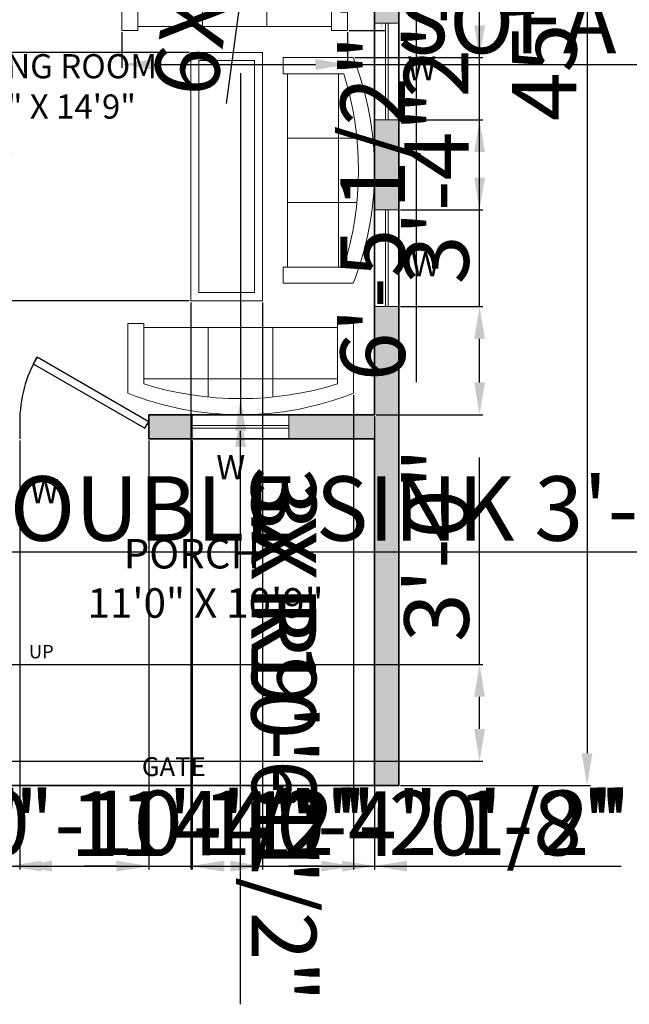
# Model space of a CAD drawing. Units: inches. Extents: x 830 to 1639, y 2591 to 3595.
# Tile 2 of 7: x 1141 to 1367, y 2591 to 2957. Entities that reach past the tile are written whole.
import ezdxf

# ---------------------------------------------------------------- set-up
doc = ezdxf.new("R2010")
doc.units = ezdxf.units.IN
doc.layers.get('0').update_dxf_attribs({"color": 250})
for name, color, linetype, lineweight in [('A-ANNO-DIMS', 2, 'Continuous', 18), ('A-ANNO-TEXT', 7, 'Continuous', 18), ('A-AREA-IDEN', 7, 'Continuous', 25), ('A-DOOR', 3, 'Continuous', 25), ('A-FURN', 8, 'Continuous', 18), ('A-GLAZ', 4, 'Continuous', 18), ('A-WALL', 7, 'Continuous', 35), ('A-WALL-PATT', 5, 'Continuous', 13), ('C-PROP', 7, 'Continuous', 35)]:
    doc.layers.add(name, color=color, linetype=linetype, lineweight=lineweight)
doc.styles.get("Standard").update_dxf_attribs({"font": 'arial.ttf'})
doc.dimstyles.new('ISO-25', dxfattribs={"dimtxt": 24, "dimasz": 12, "dimexe": 1.25, "dimexo": 0.625, "dimtad": 1, "dimdec": 0, "dimlunit": 3, "dimtxsty": 'Standard', "dimcen": 2.5, "dimadec": 0, "dimazin": 0, "dimtfac": 1, "dimtdec": 0, "dimtmove": 0, "dimatfit": 3, "dimfxl": 1, "dimarcsym": 0})

# ---------------------------------------------------------------- blocks, each defined once
blk = doc.blocks.new('Sofa - Roundback 7 ft.')
for p, q in [((-12.00002, -32.4421), (-12.00003, -6.5971)), ((11.99997, -32.4421), (11.99998, -6.5971)), ((-36.000027, -34), (-36.000027, -11.4696)), ((-35.999844, -13.3819), (35.9998, -13.3819)), ((35.99998, -34), (35.99998, -11.4696)), ((-36.000027, -32.4421), (35.99998, -32.4421))]:
    blk.add_line(p, q)
for points in [[(-36.000027, -34), (-42.000027, -34), (-42.000027, -8)], [(41.99998, -8), (41.99998, -34), (35.99998, -34)]]:
    blk.add_lwpolyline(points)
for centre, radius, start, end in [((0, -114.25), 114.25, 68.43141, 111.5686), ((-0.00001, -127.1968), 121.1968, 72.72033, 107.2797)]:
    blk.add_arc(centre, radius, start, end)
blk = doc.blocks.new('*U9')
for p, q in [((-750, 0), (-750, -100)), ((0, 0), (0, -100))]:
    blk.add_line(p, q)
blk.add_lwpolyline([(0, 0), (-649.5, 375), (-671.4, 337.1), (-21.9, -37.9)], close=True)
blk.add_arc((0, 0), 750, 150, 180)
blk = doc.blocks.new('*D14')
at = {"layer": 'A-ANNO-DIMS', "color": 0, "lineweight": -2, "transparency": 16777216}
for p, q in [((1282.21, 3212.09), (1352.88, 3212.09)), ((1351.63, 3200.09), (1351.63, 2684.09)), ((1282.21, 2672.09), (1352.88, 2672.09))]:
    blk.add_line(p, q, dxfattribs=at)
at = {"layer": 'A-ANNO-DIMS', "color": 0, "transparency": 16777216}
for points in [[(1349.63, 3200.09), (1353.63, 3200.09), (1351.63, 3212.09)], [(1349.63, 2684.09), (1353.63, 2684.09), (1351.63, 2672.09)]]:
    blk.add_solid(points, dxfattribs=at)
at = {"layer": 'Defpoints', "color": 0, "transparency": 16777216}
for p in [(1281.59, 3212.09), (1281.59, 2672.09), (1351.63, 2672.09)]:
    blk.add_point(p, dxfattribs=at)
at = {"layer": 'A-ANNO-DIMS', "color": 0, "transparency": 16777216, "insert": (1338.8, 2942.09), "char_height": 24, "attachment_point": 5, "rotation": 90}
blk.add_mtext("45'", dxfattribs=at)
blk = doc.blocks.new('WIN-36IN')
for p, q in [((0, 0), (0, 36)), ((0, 36), (9, 36)), ((4, 0), (4, 36)), ((5, 36), (5, 0)), ((9, 36), (9, 0)), ((9, 0), (0, 0))]:
    blk.add_line(p, q)
blk = doc.blocks.new('*D28')
at = {"layer": 'A-ANNO-DIMS', "color": 0, "lineweight": -2, "transparency": 16777216}
for p, q in [((1178.57, 2952.46), (1178.57, 2939.24)), ((1262.57, 2952.46), (1262.57, 2939.24)), ((1190.57, 2940.49), (1250.57, 2940.49)), ((1262.57, 2940.49), (1522.6, 2940.49))]:
    blk.add_line(p, q, dxfattribs=at)
at = {"layer": 'A-ANNO-DIMS', "color": 0, "transparency": 16777216}
for points in [[(1190.57, 2942.49), (1190.57, 2938.49), (1178.57, 2940.49)], [(1250.57, 2942.49), (1250.57, 2938.49), (1262.57, 2940.49)]]:
    blk.add_solid(points, dxfattribs=at)
at = {"layer": 'Defpoints', "color": 0, "transparency": 16777216}
for p in [(1178.57, 2953.09), (1262.57, 2953.09), (1262.57, 2940.49)]:
    blk.add_point(p, dxfattribs=at)
at = {"layer": 'A-ANNO-DIMS', "color": 0, "transparency": 16777216, "insert": (1398.58, 2953.53), "char_height": 24, "attachment_point": 5}
blk.add_mtext('SOFA 7\'-0" TYP.', dxfattribs=at)
blk = doc.blocks.new('*D29')
at = {"layer": 'A-ANNO-DIMS', "color": 0, "lineweight": -2, "transparency": 16777216}
for p, q in [((1275.17, 2989.75), (1275.17, 3205.2)), ((1263.19, 2989.75), (1276.42, 2989.75)), ((1275.17, 2965.09), (1275.17, 2977.75)), ((1263.19, 2953.09), (1276.42, 2953.09))]:
    blk.add_line(p, q, dxfattribs=at)
at = {"layer": 'A-ANNO-DIMS', "color": 0, "transparency": 16777216}
for points in [[(1273.17, 2977.75), (1277.17, 2977.75), (1275.17, 2989.75)], [(1273.17, 2965.09), (1277.17, 2965.09), (1275.17, 2953.09)]]:
    blk.add_solid(points, dxfattribs=at)
at = {"layer": 'Defpoints', "color": 0, "transparency": 16777216}
for p in [(1262.57, 2989.75), (1275.17, 2989.75), (1262.57, 2953.09)]:
    blk.add_point(p, dxfattribs=at)
at = {"layer": 'A-ANNO-DIMS', "color": 0, "transparency": 16777216, "insert": (1262.13, 3103.48), "char_height": 24, "attachment_point": 5, "rotation": 90}
blk.add_mtext('3\'-0 1/2" TYP.', dxfattribs=at)
blk = doc.blocks.new('*D37')
at = {"layer": 'A-ANNO-DIMS', "color": 0, "lineweight": -2, "transparency": 16777216}
for p, q in [((1273.21, 3115.15), (1289.3, 3115.15)), ((1288.05, 3103.15), (1288.05, 3049.83)), ((1273.21, 3037.83), (1289.3, 3037.83)), ((1288.05, 3037.83), (1288.05, 2822.23))]:
    blk.add_line(p, q, dxfattribs=at)
at = {"layer": 'A-ANNO-DIMS', "color": 0, "transparency": 16777216}
for points in [[(1286.05, 3103.15), (1290.05, 3103.15), (1288.05, 3115.15)], [(1286.05, 3049.83), (1290.05, 3049.83), (1288.05, 3037.83)]]:
    blk.add_solid(points, dxfattribs=at)
at = {"layer": 'Defpoints', "color": 0, "transparency": 16777216}
for p in [(1272.59, 3115.15), (1272.59, 3037.83), (1288.05, 3037.83)]:
    blk.add_point(p, dxfattribs=at)
at = {"layer": 'A-ANNO-DIMS', "color": 0, "transparency": 16777216, "insert": (1275.02, 2924.03), "char_height": 24, "attachment_point": 5, "rotation": 90}
blk.add_mtext('6\'-5 1/2" TYP.', dxfattribs=at)
blk = doc.blocks.new('*D42')
at = {"layer": 'A-ANNO-DIMS', "color": 0, "lineweight": -2, "transparency": 16777216}
for p, q in [((1062.05, 2763.79), (1062.05, 2757.77)), ((1098.05, 2763.79), (1098.05, 2757.77)), ((1074.05, 2759.02), (1086.05, 2759.02)), ((1098.05, 2759.02), (1408.67, 2759.02))]:
    blk.add_line(p, q, dxfattribs=at)
at = {"layer": 'A-ANNO-DIMS', "color": 0, "transparency": 16777216}
for points in [[(1074.05, 2761.02), (1074.05, 2757.02), (1062.05, 2759.02)], [(1086.05, 2761.02), (1086.05, 2757.02), (1098.05, 2759.02)]]:
    blk.add_solid(points, dxfattribs=at)
at = {"layer": 'Defpoints', "color": 0, "transparency": 16777216}
for p in [(1062.05, 2764.42), (1098.05, 2764.42), (1098.05, 2759.02)]:
    blk.add_point(p, dxfattribs=at)
at = {"layer": 'A-ANNO-DIMS', "color": 0, "transparency": 16777216, "insert": (1259.36, 2772.07), "char_height": 24, "attachment_point": 5}
blk.add_mtext('DOUBLE SINK 3\'-0"', dxfattribs=at)
blk = doc.blocks.new('*D46')
at = {"layer": 'A-ANNO-DIMS', "color": 0, "lineweight": -2, "transparency": 16777216}
for p, q in [((1136.59, 2671.46), (1136.59, 2640.79)), ((1272.59, 2671.46), (1272.59, 2640.79)), ((1148.59, 2642.04), (1260.59, 2642.04))]:
    blk.add_line(p, q, dxfattribs=at)
at = {"layer": 'A-ANNO-DIMS', "color": 0, "transparency": 16777216}
for points in [[(1148.59, 2644.04), (1148.59, 2640.04), (1136.59, 2642.04)], [(1260.59, 2644.04), (1260.59, 2640.04), (1272.59, 2642.04)]]:
    blk.add_solid(points, dxfattribs=at)
at = {"layer": 'Defpoints', "color": 0, "transparency": 16777216}
for p in [(1136.59, 2672.09), (1272.59, 2672.09), (1272.59, 2642.04)]:
    blk.add_point(p, dxfattribs=at)
at = {"layer": 'A-ANNO-DIMS', "color": 0, "transparency": 16777216, "insert": (1204.59, 2654.71), "char_height": 24, "attachment_point": 5}
blk.add_mtext('11\'-4"', dxfattribs=at)
blk = doc.blocks.new('*D48')
at = {"layer": 'A-ANNO-DIMS', "color": 0, "lineweight": -2, "transparency": 16777216}
for p, q in [((1140.59, 2800.46), (1140.59, 2640.79)), ((1188.59, 2800.46), (1188.59, 2640.79)), ((1152.59, 2642.04), (1176.59, 2642.04)), ((1188.59, 2642.04), (1266.6, 2642.04))]:
    blk.add_line(p, q, dxfattribs=at)
at = {"layer": 'A-ANNO-DIMS', "color": 0, "transparency": 16777216}
for points in [[(1152.59, 2644.04), (1152.59, 2640.04), (1140.59, 2642.04)], [(1176.59, 2644.04), (1176.59, 2640.04), (1188.59, 2642.04)]]:
    blk.add_solid(points, dxfattribs=at)
at = {"layer": 'Defpoints', "color": 0, "transparency": 16777216}
for p in [(1140.59, 2801.09), (1188.59, 2801.09), (1188.59, 2642.04)]:
    blk.add_point(p, dxfattribs=at)
at = {"layer": 'A-ANNO-DIMS', "color": 0, "transparency": 16777216, "insert": (1233.6, 2654.92), "char_height": 24, "attachment_point": 5}
blk.add_mtext('4\'-0"', dxfattribs=at)
blk = doc.blocks.new('*D53')
at = {"layer": 'A-ANNO-DIMS', "color": 0, "lineweight": -2, "transparency": 16777216}
for p, q in [((1026.59, 2680.46), (1026.59, 2640.79)), ((1036.59, 2680.46), (1036.59, 2640.79)), ((1014.59, 2642.04), (1002.59, 2642.04)), ((1026.59, 2642.04), (1036.59, 2642.04)), ((1048.59, 2642.04), (1144.28, 2642.04))]:
    blk.add_line(p, q, dxfattribs=at)
at = {"layer": 'A-ANNO-DIMS', "color": 0, "transparency": 16777216}
for points in [[(1014.59, 2644.04), (1014.59, 2640.04), (1026.59, 2642.04)], [(1048.59, 2644.04), (1048.59, 2640.04), (1036.59, 2642.04)]]:
    blk.add_solid(points, dxfattribs=at)
at = {"layer": 'Defpoints', "color": 0, "transparency": 16777216}
for p in [(1026.59, 2681.09), (1036.59, 2681.09), (1036.59, 2642.04)]:
    blk.add_point(p, dxfattribs=at)
at = {"layer": 'A-ANNO-DIMS', "color": 0, "transparency": 16777216, "insert": (1102.44, 2654.92), "char_height": 24, "attachment_point": 5}
blk.add_mtext('0\'-10"', dxfattribs=at)
blk = doc.blocks.new('*D55')
at = {"layer": 'A-ANNO-DIMS', "color": 0, "lineweight": -2, "transparency": 16777216}
for p, q in [((1311.64, 2717.09), (1311.64, 2794.12)), ((1137.21, 2717.09), (1312.89, 2717.09)), ((1311.64, 2693.09), (1311.64, 2705.09)), ((1137.21, 2681.09), (1312.89, 2681.09))]:
    blk.add_line(p, q, dxfattribs=at)
at = {"layer": 'A-ANNO-DIMS', "color": 0, "transparency": 16777216}
for points in [[(1309.64, 2705.09), (1313.64, 2705.09), (1311.64, 2717.09)], [(1309.64, 2693.09), (1313.64, 2693.09), (1311.64, 2681.09)]]:
    blk.add_solid(points, dxfattribs=at)
at = {"layer": 'Defpoints', "color": 0, "transparency": 16777216}
for p in [(1136.59, 2717.09), (1311.64, 2717.09), (1136.59, 2681.09)]:
    blk.add_point(p, dxfattribs=at)
at = {"layer": 'A-ANNO-DIMS', "color": 0, "transparency": 16777216, "insert": (1298.75, 2761.6), "char_height": 24, "attachment_point": 5, "rotation": 90}
blk.add_mtext('3\'-0"', dxfattribs=at)
blk = doc.blocks.new('*D56')
at = {"layer": 'A-ANNO-DIMS', "color": 0, "lineweight": -2, "transparency": 16777216}
for p, q in [((1204.22, 2851.9), (1204.22, 2640.79)), ((1230.9, 2851.9), (1230.9, 2640.79)), ((1216.22, 2642.04), (1218.9, 2642.04)), ((1230.9, 2642.04), (1364.28, 2642.04))]:
    blk.add_line(p, q, dxfattribs=at)
at = {"layer": 'A-ANNO-DIMS', "color": 0, "transparency": 16777216}
for points in [[(1216.22, 2644.04), (1216.22, 2640.04), (1204.22, 2642.04)], [(1218.9, 2644.04), (1218.9, 2640.04), (1230.9, 2642.04)]]:
    blk.add_solid(points, dxfattribs=at)
at = {"layer": 'Defpoints', "color": 0, "transparency": 16777216}
for p in [(1204.22, 2852.53), (1230.9, 2852.53), (1230.9, 2642.04)]:
    blk.add_point(p, dxfattribs=at)
at = {"layer": 'A-ANNO-DIMS', "color": 0, "transparency": 16777216, "insert": (1303.59, 2655.07), "char_height": 24, "attachment_point": 5}
blk.add_mtext('2\'-2 1/2"', dxfattribs=at)
blk = doc.blocks.new('*D57')
at = {"layer": 'A-ANNO-DIMS', "color": 0, "lineweight": -2, "transparency": 16777216}
for p, q in [((951.54, 2944.9), (951.54, 3077.67)), ((1203.59, 2944.9), (950.29, 2944.9)), ((951.54, 2864.53), (951.54, 2932.9)), ((1203.59, 2852.53), (950.29, 2852.53))]:
    blk.add_line(p, q, dxfattribs=at)
at = {"layer": 'A-ANNO-DIMS', "color": 0, "transparency": 16777216}
for points in [[(949.54, 2932.9), (953.54, 2932.9), (951.54, 2944.9)], [(949.54, 2864.53), (953.54, 2864.53), (951.54, 2852.53)]]:
    blk.add_solid(points, dxfattribs=at)
at = {"layer": 'Defpoints', "color": 0, "transparency": 16777216}
for p in [(951.54, 2944.9), (1204.22, 2944.9), (1204.22, 2852.53)]:
    blk.add_point(p, dxfattribs=at)
at = {"layer": 'A-ANNO-DIMS', "color": 0, "transparency": 16777216, "insert": (938.51, 3017.28), "char_height": 24, "attachment_point": 5, "rotation": 90}
blk.add_mtext('7\'-8 1/2"', dxfattribs=at)
blk = doc.blocks.new('*D62')
at = {"layer": 'A-ANNO-DIMS', "color": 0, "lineweight": -2, "transparency": 16777216}
for p, q in [((1311.64, 2850.33), (1311.64, 2927.36)), ((1282.21, 2850.33), (1312.89, 2850.33)), ((1311.64, 2822.09), (1311.64, 2838.33)), ((1273.21, 2810.09), (1312.89, 2810.09))]:
    blk.add_line(p, q, dxfattribs=at)
at = {"layer": 'A-ANNO-DIMS', "color": 0, "transparency": 16777216}
for points in [[(1309.64, 2838.33), (1313.64, 2838.33), (1311.64, 2850.33)], [(1309.64, 2822.09), (1313.64, 2822.09), (1311.64, 2810.09)]]:
    blk.add_solid(points, dxfattribs=at)
at = {"layer": 'Defpoints', "color": 0, "transparency": 16777216}
for p in [(1281.59, 2850.33), (1311.64, 2850.33), (1272.59, 2810.09)]:
    blk.add_point(p, dxfattribs=at)
at = {"layer": 'A-ANNO-DIMS', "color": 0, "transparency": 16777216, "insert": (1298.75, 2894.84), "char_height": 24, "attachment_point": 5, "rotation": 90}
blk.add_mtext('3\'-4"', dxfattribs=at)
blk = doc.blocks.new('*D63')
at = {"layer": 'A-ANNO-DIMS', "color": 0, "lineweight": -2, "transparency": 16777216}
for p, q in [((1311.64, 2919.85), (1311.64, 3053.23)), ((1282.21, 2919.85), (1312.89, 2919.85)), ((1311.64, 2898.33), (1311.64, 2907.85)), ((1282.21, 2886.33), (1312.89, 2886.33))]:
    blk.add_line(p, q, dxfattribs=at)
at = {"layer": 'A-ANNO-DIMS', "color": 0, "transparency": 16777216}
for points in [[(1309.64, 2907.85), (1313.64, 2907.85), (1311.64, 2919.85)], [(1309.64, 2898.33), (1313.64, 2898.33), (1311.64, 2886.33)]]:
    blk.add_solid(points, dxfattribs=at)
at = {"layer": 'Defpoints', "color": 0, "transparency": 16777216}
for p in [(1281.59, 2919.85), (1311.64, 2919.85), (1281.59, 2886.33)]:
    blk.add_point(p, dxfattribs=at)
at = {"layer": 'A-ANNO-DIMS', "color": 0, "transparency": 16777216, "insert": (1298.61, 2992.54), "char_height": 24, "attachment_point": 5, "rotation": 90}
blk.add_mtext('2\'-9 1/2"', dxfattribs=at)
blk = doc.blocks.new('*D64')
at = {"layer": 'A-ANNO-DIMS', "color": 0, "lineweight": -2, "transparency": 16777216}
for p, q in [((1095.59, 2895.07), (1095.59, 2640.79)), ((1105.88, 2895.07), (1105.88, 2640.79)), ((1083.59, 2642.04), (1071.59, 2642.04)), ((1095.59, 2642.04), (1105.88, 2642.04)), ((1117.88, 2642.04), (1269.5, 2642.04))]:
    blk.add_line(p, q, dxfattribs=at)
at = {"layer": 'A-ANNO-DIMS', "color": 0, "transparency": 16777216}
for points in [[(1083.59, 2644.04), (1083.59, 2640.04), (1095.59, 2642.04)], [(1117.88, 2644.04), (1117.88, 2640.04), (1105.88, 2642.04)]]:
    blk.add_solid(points, dxfattribs=at)
at = {"layer": 'Defpoints', "color": 0, "transparency": 16777216}
for p in [(1095.59, 2895.7), (1105.88, 2895.7), (1105.88, 2642.04)]:
    blk.add_point(p, dxfattribs=at)
at = {"layer": 'A-ANNO-DIMS', "color": 0, "transparency": 16777216, "insert": (1199.69, 2655.07), "char_height": 24, "attachment_point": 5}
blk.add_mtext('0\'-10 1/2"', dxfattribs=at)
blk = doc.blocks.new('*D65')
at = {"layer": 'A-ANNO-DIMS', "color": 0, "lineweight": -2, "transparency": 16777216}
for p, q in [((1106.51, 2953.33), (1137.18, 2953.33)), ((1135.93, 2941.33), (1135.93, 2907.7)), ((1106.51, 2895.7), (1137.18, 2895.7)), ((1135.93, 2895.7), (1135.93, 2761.76))]:
    blk.add_line(p, q, dxfattribs=at)
at = {"layer": 'A-ANNO-DIMS', "color": 0, "transparency": 16777216}
for points in [[(1133.93, 2941.33), (1137.93, 2941.33), (1135.93, 2953.33)], [(1133.93, 2907.7), (1137.93, 2907.7), (1135.93, 2895.7)]]:
    blk.add_solid(points, dxfattribs=at)
at = {"layer": 'Defpoints', "color": 0, "transparency": 16777216}
for p in [(1105.88, 2953.33), (1105.88, 2895.7), (1135.93, 2895.7)]:
    blk.add_point(p, dxfattribs=at)
at = {"layer": 'A-ANNO-DIMS', "color": 0, "transparency": 16777216, "insert": (1122.9, 2822.73), "char_height": 24, "attachment_point": 5, "rotation": 90}
blk.add_mtext('4\'-9 1/2"', dxfattribs=at)
blk = doc.blocks.new('*D66')
at = {"layer": 'A-ANNO-DIMS', "color": 0, "lineweight": -2, "transparency": 16777216}
for p, q in [((1264.75, 2817.46), (1264.75, 2640.79)), ((1272.59, 2809.46), (1272.59, 2640.79)), ((1252.75, 2642.04), (1240.75, 2642.04)), ((1264.75, 2642.04), (1272.59, 2642.04)), ((1284.59, 2642.04), (1361.64, 2642.04))]:
    blk.add_line(p, q, dxfattribs=at)
at = {"layer": 'A-ANNO-DIMS', "color": 0, "transparency": 16777216}
for points in [[(1252.75, 2644.04), (1252.75, 2640.04), (1264.75, 2642.04)], [(1284.59, 2644.04), (1284.59, 2640.04), (1272.59, 2642.04)]]:
    blk.add_solid(points, dxfattribs=at)
at = {"layer": 'Defpoints', "color": 0, "transparency": 16777216}
for p in [(1264.75, 2818.09), (1272.59, 2810.09), (1272.59, 2642.04)]:
    blk.add_point(p, dxfattribs=at)
at = {"layer": 'A-ANNO-DIMS', "color": 0, "transparency": 16777216, "insert": (1329.11, 2654.92), "char_height": 24, "attachment_point": 5}
blk.add_mtext('0\'-8"', dxfattribs=at)
blk = doc.blocks.new('*D67')
at = {"layer": 'A-ANNO-DIMS', "color": 0, "lineweight": -2, "transparency": 16777216}
for p, q in [((1311.64, 2987.09), (1311.64, 3064.12)), ((1273.21, 2987.09), (1312.89, 2987.09)), ((1311.64, 2955.04), (1311.64, 2975.09)), ((1265.21, 2943.04), (1312.89, 2943.04))]:
    blk.add_line(p, q, dxfattribs=at)
at = {"layer": 'A-ANNO-DIMS', "color": 0, "transparency": 16777216}
for points in [[(1309.64, 2975.09), (1313.64, 2975.09), (1311.64, 2987.09)], [(1309.64, 2955.04), (1313.64, 2955.04), (1311.64, 2943.04)]]:
    blk.add_solid(points, dxfattribs=at)
at = {"layer": 'Defpoints', "color": 0, "transparency": 16777216}
for p in [(1272.59, 2987.09), (1311.64, 2987.09), (1264.59, 2943.04)]:
    blk.add_point(p, dxfattribs=at)
at = {"layer": 'A-ANNO-DIMS', "color": 0, "transparency": 16777216, "insert": (1298.75, 3031.6), "char_height": 24, "attachment_point": 5, "rotation": 90}
blk.add_mtext('3\'-8"', dxfattribs=at)
blk = doc.blocks.new('*D72')
at = {"layer": 'A-ANNO-DIMS', "color": 0, "lineweight": -2, "transparency": 16777216}
for p, q in [((1188.59, 2800.46), (1188.59, 2640.79)), ((1204.75, 2800.46), (1204.75, 2640.79)), ((1176.59, 2642.04), (1164.59, 2642.04)), ((1188.59, 2642.04), (1204.75, 2642.04)), ((1216.75, 2642.04), (1291.54, 2642.04))]:
    blk.add_line(p, q, dxfattribs=at)
at = {"layer": 'A-ANNO-DIMS', "color": 0, "transparency": 16777216}
for points in [[(1176.59, 2644.04), (1176.59, 2640.04), (1188.59, 2642.04)], [(1216.75, 2644.04), (1216.75, 2640.04), (1204.75, 2642.04)]]:
    blk.add_solid(points, dxfattribs=at)
at = {"layer": 'Defpoints', "color": 0, "transparency": 16777216}
for p in [(1188.59, 2801.09), (1204.75, 2801.09), (1204.75, 2642.04)]:
    blk.add_point(p, dxfattribs=at)
at = {"layer": 'A-ANNO-DIMS', "color": 0, "transparency": 16777216, "insert": (1260.15, 2654.71), "char_height": 24, "attachment_point": 5}
blk.add_mtext('1\'-4"', dxfattribs=at)
blk = doc.blocks.new('*D73')
at = {"layer": 'A-ANNO-DIMS', "color": 0, "lineweight": -2, "transparency": 16777216}
for p, q in [((1222.75, 2937.28), (1222.76, 2816.09)), ((1222.76, 2633.87), (1222.76, 2804.09))]:
    blk.add_line(p, q, dxfattribs=at)
at = {"layer": 'A-ANNO-DIMS', "color": 0, "transparency": 16777216}
blk.add_solid([(1224.76, 2804.09), (1220.76, 2804.09), (1222.76, 2816.09)], dxfattribs=at)
at = {"layer": 'Defpoints', "color": 0, "transparency": 16777216}
for p in [(1222.75, 2937.28), (1222.76, 2816.09)]:
    blk.add_point(p, dxfattribs=at)
at = {"layer": 'A-ANNO-DIMS', "color": 0, "transparency": 16777216, "insert": (1235.64, 2712.98), "char_height": 24, "attachment_point": 5, "rotation": 270.0002}
blk.add_mtext('3X R10\'-1"', dxfattribs=at)
blk = doc.blocks.new('*D74')
at = {"layer": 'A-ANNO-DIMS', "color": 0, "lineweight": -2, "transparency": 16777216}
for p, q in [((1222.75, 2924.34), (1222.76, 2810.09)), ((1222.76, 2590.59), (1222.76, 2798.09))]:
    blk.add_line(p, q, dxfattribs=at)
at = {"layer": 'A-ANNO-DIMS', "color": 0, "transparency": 16777216}
blk.add_solid([(1224.76, 2798.09), (1220.76, 2798.09), (1222.76, 2810.09)], dxfattribs=at)
at = {"layer": 'Defpoints', "color": 0, "transparency": 16777216}
for p in [(1222.75, 2924.34), (1222.76, 2810.09)]:
    blk.add_point(p, dxfattribs=at)
at = {"layer": 'A-ANNO-DIMS', "color": 0, "transparency": 16777216, "insert": (1235.8, 2688.34), "char_height": 24, "attachment_point": 5, "rotation": 270.0002}
blk.add_mtext('3X R9\'-6 1/2"', dxfattribs=at)
blk = doc.blocks.new('*D76')
at = {"layer": 'A-ANNO-DIMS', "color": 0, "lineweight": -2, "transparency": 16777216}
for p, q in [((1250.77, 3173.28), (1249.26, 3162.05)), ((1217.52, 2925.89), (1247.66, 3150.16))]:
    blk.add_line(p, q, dxfattribs=at)
at = {"layer": 'A-ANNO-DIMS', "color": 0, "transparency": 16777216}
blk.add_solid([(1245.68, 3150.42), (1249.65, 3149.89), (1249.26, 3162.05)], dxfattribs=at)
at = {"layer": 'Defpoints', "color": 0, "transparency": 16777216}
for p in [(1250.77, 3173.28), (1249.26, 3162.05)]:
    blk.add_point(p, dxfattribs=at)
at = {"layer": 'A-ANNO-DIMS', "color": 0, "transparency": 16777216, "insert": (1218.87, 3033.81), "char_height": 24, "attachment_point": 5, "rotation": 82.3443}
blk.add_mtext('6X R0\'-11 1/2"', dxfattribs=at)

msp = doc.modelspace()

# ---------------------------------------------------------------- hatches: boundary and pattern name
at = {"layer": 'A-WALL-PATT'}
h = msp.add_hatch(color=256, dxfattribs=at)
h.dxf.hatch_style = 1
h.paths.add_polyline_path([(1281.59, 3058.42), (1272.59, 3058.42), (1272.59, 3037.83), (1272.63, 3037.83), (1272.63, 3018.58), (1272.59, 2991.09), (1176.59, 2991.09), (1176.59, 2987.09), (1272.59, 2987.09), (1272.59, 2955.85), (1281.59, 2955.85)])
h = msp.add_hatch(color=256, dxfattribs=at)
h.dxf.hatch_style = 1
h.paths.add_polyline_path([(1272.59, 2886.33), (1281.59, 2886.33), (1281.59, 2919.85), (1272.59, 2919.85)])
h = msp.add_hatch(color=256, dxfattribs=at)
h.dxf.hatch_style = 1
h.paths.add_polyline_path([(1281.59, 2850.33), (1272.59, 2850.33), (1272.59, 2810.09), (1240.75, 2810.09), (1240.75, 2801.09), (1272.59, 2801.09), (1272.59, 2672.09), (1281.59, 2672.09)])
h = msp.add_hatch(color=256, dxfattribs=at)
h.dxf.hatch_style = 1
h.paths.add_polyline_path([(1188.59, 2810.09), (1188.59, 2801.09), (1204.75, 2801.09), (1204.75, 2810.09)])

# ---------------------------------------------------------------- linework, layer by layer
at = {"layer": 'A-FURN'}
for points in [[(1204.22, 2944.9), (1230.9, 2944.9), (1230.9, 2852.53), (1204.22, 2852.53)], [(1207.22, 2941.9), (1227.9, 2941.9), (1227.9, 2855.53), (1207.22, 2855.53)]]:
    msp.add_lwpolyline(points, close=True, dxfattribs=at)
at = {"layer": 'A-WALL'}
for p, q in [((1272.59, 2987.09), (1272.59, 2810.09)), ((1272.59, 2810.09), (1272.59, 2987.09)), ((1188.59, 2801.09), (1188.59, 2810.09)), ((1188.59, 2810.09), (1272.59, 2810.09)), ((1188.59, 2801.09), (1272.59, 2801.09)), ((1272.59, 2672.09), (1272.59, 2801.09)), ((1272.59, 2801.09), (1272.59, 2681.09))]:
    msp.add_line(p, q, dxfattribs=at)
at = {"layer": 'C-PROP'}
msp.add_line((981.59, 2672.09), (1281.59, 2672.09), dxfattribs=at)
msp.add_lwpolyline([(981.59, 3212.09), (1281.59, 3212.09), (1281.59, 2672.09), (981.59, 2672.09)], close=True, dxfattribs=at)

# ---------------------------------------------------------------- block references
at = {"layer": 'A-DOOR', "xscale": 0.0639999999999998, "yscale": 0.0639999999999998, "zscale": 0.0639999999999998}
msp.add_blockref('*U9', (1188.59, 2807.49), dxfattribs=at)
at = {"layer": 'A-FURN'}
msp.add_blockref('Sofa - Roundback 7 ft.', (1220.57, 2987.09), dxfattribs=at)
for p, rotation in [((1272.59, 2901.04), 270), ((1222.75, 2810.09), 180)]:
    msp.add_blockref('Sofa - Roundback 7 ft.', p, dxfattribs=dict(at, rotation=rotation))
at = {"layer": 'A-GLAZ'}
for p in [(1272.59, 2919.85), (1272.59, 2850.33)]:
    msp.add_blockref('WIN-36IN', p, dxfattribs=at)
at = {"layer": 'A-GLAZ', "rotation": 269.9999999999966}
msp.add_blockref('WIN-36IN', (1204.75, 2810.09), dxfattribs=at)

# ---------------------------------------------------------------- texts
at = {"layer": 'A-ANNO-TEXT', "char_height": 9, "width": 31.3961, "attachment_point": 1}
for insert in [(1284.73, 2943.54), (1286.12, 2870.62), (1213.71, 2795.07), (1144.4, 2786.12)]:
    msp.add_mtext('{\\fArial|b1|i0|c0|p34;W}', dxfattribs=dict(at, insert=insert))
at = {"layer": 'A-ANNO-TEXT', "attachment_point": 1}
for s, width, heights, insert, char_height in [('{\\fArial|b1|i0|c0|p34;UP}', 75.9739, [2.5], (1144, 2724.39), 5), ('{\\fArial|b1|i0|c0|p34;GATE}', 78.5758, [0], (1186.03, 2682.57), 7)]:
    msp.add_mtext_dynamic_manual_height_columns(s, width=width, gutter_width=12.5, heights=heights, dxfattribs=dict(at, insert=insert, char_height=char_height))
at = {"layer": 'A-AREA-IDEN', "insert": (1111.93, 2944.33), "char_height": 9, "attachment_point": 1}
msp.add_mtext_dynamic_manual_height_columns('{\\fArial|b1|i0|c0|p34; LIVING ROOM\\P14\'9" X 14\'9"}', width=90.0444, gutter_width=12.5, heights=[67], dxfattribs=at)
at = {"layer": 'A-AREA-IDEN', "insert": (1165.83, 2763.84), "char_height": 11, "width": 123.0713, "attachment_point": 1}
msp.add_mtext('{\\fArial|b1|i0|c0|p34;    PORCH \\P11\'0" X 10\'9"}', dxfattribs=at)

# ---------------------------------------------------------------- dimensions: what is measured, and where the dimension line sits
at = {"layer": 'A-ANNO-DIMS'}
for base, p1, p2, angle, override, picture, middle in [((1351.63, 2672.09), (1281.59, 3212.09), (1281.59, 2672.09), 90, {"dimclrd": 0, "dimclre": 0, "dimclrt": 0}, '*D14', (1338.8, 2942.09)), ((951.54, 2944.9), (1204.22, 2852.53), (1204.22, 2944.9), 90, {"dimdec": 1, "dimlfac": 1, "dimrnd": 0, "dimzin": 1, "dimdsep": 46, "dimlunit": 4, "dimfrac": 2}, '*D57', (938.51, 3017.28)), ((1311.6397, 2987.0874), (1264.5897, 2943.038), (1272.5897, 2987.0874), 90, {"dimdec": 1, "dimlfac": 1, "dimrnd": 0, "dimzin": 1, "dimdsep": 46, "dimlunit": 4, "dimfrac": 2}, '*D67', (1298.7528, 3031.6033)), ((1311.64, 2919.85), (1281.59, 2886.33), (1281.59, 2919.85), 90, {"dimdec": 1, "dimlfac": 1, "dimrnd": 0, "dimzin": 1, "dimdsep": 46, "dimlunit": 4, "dimfrac": 2}, '*D63', (1298.61, 2992.54)), ((1135.93, 2895.7), (1105.88, 2953.33), (1105.88, 2895.7), 270, {"dimdec": 1, "dimlfac": 1, "dimrnd": 0, "dimzin": 1, "dimdsep": 46, "dimlunit": 4, "dimfrac": 2}, '*D65', (1122.9, 2822.73)), ((1311.64, 2850.33), (1272.59, 2810.09), (1281.59, 2850.33), 90, {"dimdec": 1, "dimlfac": 1, "dimrnd": 0, "dimzin": 1, "dimdsep": 46, "dimlunit": 4, "dimfrac": 2}, '*D62', (1298.75, 2894.84)), ((1311.64, 2717.09), (1136.59, 2681.09), (1136.59, 2717.09), 90, {"dimdec": 1, "dimlfac": 1, "dimrnd": 0, "dimzin": 1, "dimdsep": 46, "dimlunit": 4, "dimfrac": 2}, '*D55', (1298.75, 2761.6))]:
    dim = msp.add_linear_dim(base=base, p1=p1, p2=p2, angle=angle, dimstyle='ISO-25', override=override, dxfattribs=at)
    dim.commit()
    dim.dimension.update_dxf_attribs({"geometry": picture, "text_midpoint": middle})
for base, p1, p2, angle, picture, middle in [((1275.17, 2989.75), (1262.57, 2953.09), (1262.57, 2989.75), 90, '*D29', (1262.13, 3103.48)), ((1288.05, 3037.83), (1272.59, 3115.15), (1272.59, 3037.83), 270, '*D37', (1275.02, 2924.03))]:
    dim = msp.add_linear_dim(base=base, p1=p1, p2=p2, angle=angle, text='<> TYP.', dimstyle='ISO-25', override={"dimdec": 1, "dimlfac": 1, "dimrnd": 0, "dimzin": 1, "dimdsep": 46, "dimlunit": 4, "dimfrac": 2}, dxfattribs=at)
    dim.commit()
    dim.dimension.update_dxf_attribs({"geometry": picture, "text_midpoint": middle})
for center, mpoint, text, picture, middle in [((1250.77, 3173.28), (1249.26, 3162.05), '6X <>', '*D76', (1218.87, 3033.81)), ((1222.75, 2937.28), (1222.76, 2816.09), '3X <>', '*D73', (1235.64, 2712.98)), ((1222.75, 2924.34), (1222.76, 2810.09), '3X <>', '*D74', (1235.8, 2688.34))]:
    dim = msp.add_radius_dim(center=center, mpoint=mpoint, text=text, dimstyle='ISO-25', override={"dimdec": 1, "dimlfac": 1, "dimrnd": 0, "dimzin": 1, "dimdsep": 46, "dimlunit": 4, "dimfrac": 2}, dxfattribs=at)
    dim.commit()
    dim.dimension.update_dxf_attribs({"geometry": picture, "text_midpoint": middle})
for base, p1, p2, text, picture, middle in [((1262.57, 2940.49), (1178.57, 2953.09), (1262.57, 2953.09), 'SOFA <> TYP.', '*D28', (1398.58, 2953.53)), ((1098.05, 2759.02), (1062.05, 2764.42), (1098.05, 2764.42), 'DOUBLE SINK <>', '*D42', (1259.36, 2772.07))]:
    dim = msp.add_linear_dim(base=base, p1=p1, p2=p2, text=text, dimstyle='ISO-25', override={"dimdec": 1, "dimlfac": 1, "dimrnd": 0, "dimzin": 1, "dimdsep": 46, "dimlunit": 4, "dimfrac": 2}, dxfattribs=at)
    dim.commit()
    dim.dimension.update_dxf_attribs({"geometry": picture, "text_midpoint": middle})
for base, p1, p2, picture, middle in [((1105.88, 2642.04), (1095.59, 2895.7), (1105.88, 2895.7), '*D64', (1199.69, 2655.07)), ((1230.9, 2642.04), (1204.22, 2852.53), (1230.9, 2852.53), '*D56', (1303.59, 2655.07)), ((1272.59, 2642.04), (1264.75, 2818.09), (1272.59, 2810.09), '*D66', (1329.11, 2654.92)), ((1188.59, 2642.04), (1140.59, 2801.09), (1188.59, 2801.09), '*D48', (1233.6, 2654.92)), ((1204.75, 2642.04), (1188.59, 2801.09), (1204.75, 2801.09), '*D72', (1260.15, 2654.71)), ((1036.59, 2642.04), (1026.59, 2681.09), (1036.59, 2681.09), '*D53', (1102.44, 2654.92)), ((1272.59, 2642.04), (1136.59, 2672.09), (1272.59, 2672.09), '*D46', (1204.59, 2654.71))]:
    dim = msp.add_linear_dim(base=base, p1=p1, p2=p2, dimstyle='ISO-25', override={"dimdec": 1, "dimlfac": 1, "dimrnd": 0, "dimzin": 1, "dimdsep": 46, "dimlunit": 4, "dimfrac": 2}, dxfattribs=at)
    dim.commit()
    dim.dimension.update_dxf_attribs({"geometry": picture, "text_midpoint": middle})

doc.saveas('drawing.dxf')
